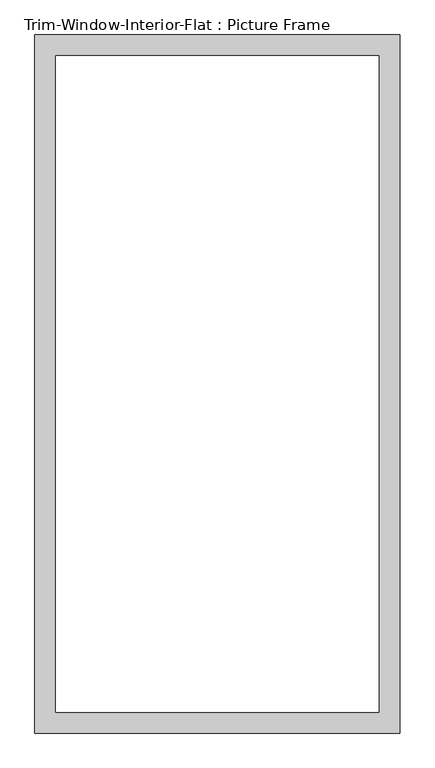
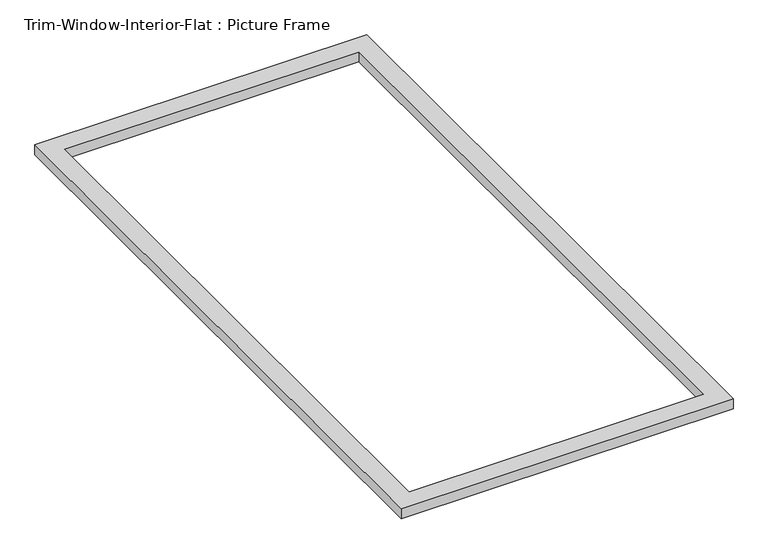
"""IFC4 building model written with IfcOpenShell, lengths in millimetres: proxy geometry, Trim-Window-Interior-Flat : Picture Frame."""

from ifc_helpers import new_model, si_unit, origin, origin_with_axes, place, context, project, spatial, polyline, outline, extrude, source, transform, mapped, element, save


def trim_window_interior_flat_picture_frame_d9cdb79e(model_context):
    return source(origin(), model_context, "Body", "SweptSolid", [
        extrude(outline(polyline([(501.65, 44.45), (501.65, -1873.25), (-501.65, -1873.25), (-501.65, 44.45), (501.65, 44.45)]), holes=[polyline([(444.5, -12.7), (-444.5, -12.7), (-444.5, -1816.1), (444.5, -1816.1), (444.5, -12.7)])]), origin_with_axes(), (0.0, 0.0, 1.0), 31.75),
    ])


if __name__ == "__main__":
    model = new_model("IFC4")
    model_context = context("Model", 3, world=origin())
    ifc_project = project(units=[si_unit("LENGTHUNIT", "METRE", prefix="MILLI")], contexts=[model_context])
    site = spatial("IfcSite", under=ifc_project)
    building = spatial("IfcBuilding", under=site)
    placement = place(None, origin())
    trim_window_interior_flat_picture_frame_shape = trim_window_interior_flat_picture_frame_d9cdb79e(model_context)
    element("IfcBuildingElementProxy", 1, Name="Trim-Window-Interior-Flat : Picture Frame", ObjectType="Trim-Window-Interior-Flat : Picture Frame", at=placement, inside=building, context=model_context, shape_type="MappedRepresentation", body=[
        mapped(trim_window_interior_flat_picture_frame_shape, transform((0.0, 0.0, 0.0), x_axis=(1.0, 0.0, 0.0), y_axis=(0.0, 1.0, 0.0), z_axis=(0.0, 0.0, 1.0))),
    ])
    save(model, "model.ifc")

# Revit data of these elements
# Type "Trim-Window-Interior-Flat : Picture Frame"
#   Trim Thickness_Picture Frame = 0' - 1 1/4"
#   Trim Width = 0' - 2 1/4"
#   Trim Thickness_with Sill = 0' - 0 3/4"
#   Sill Thickness = 0' - 1 1/4"
#   Opening Width [instance default] = 2' - 0"
#   Opening Height [instance default] = 3' - 0"
#   Default Elevation = 4' - 0"
#   Sill = no
#   Picture Frame = yes
#   Trim Material [instance default] = none
# Element 1 (IfcBuildingElementProxy, "Trim-Window-Interior-Flat : Picture Frame")
#   Opening Width = 3' - 0"
#   Opening Height = 6' - 0"
#   Trim Material = Wood - Stained
#   Materials on its faces: "Wood - Stained"
# Materials
#   "Wood - Stained": class "Wood", colour RGB 224 178 126, transparency 0, Cost = 0
